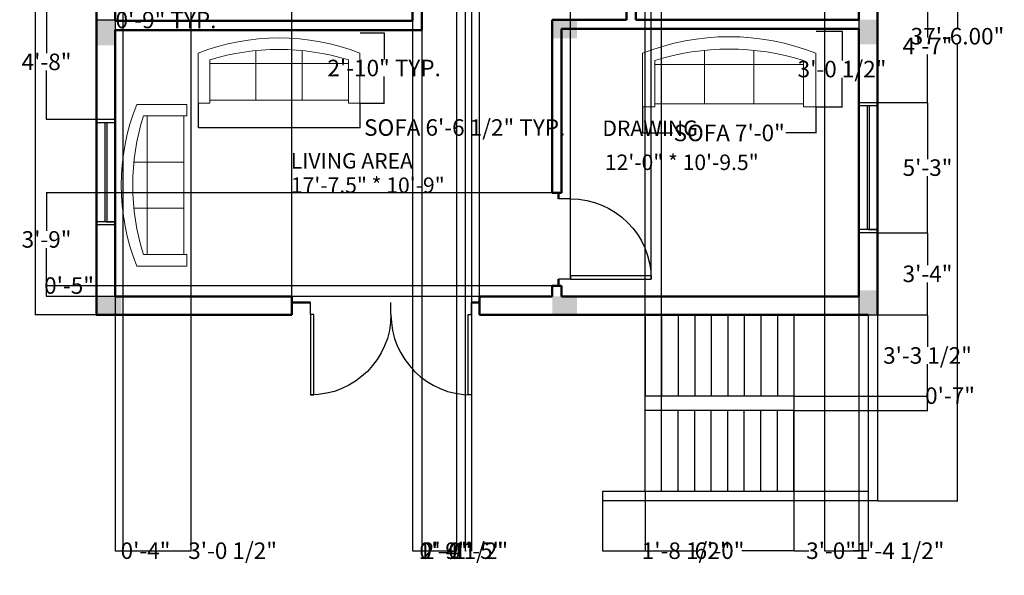
# Model space of a CAD drawing. Units: inches. Extents: x 9717 to 10218, y 17835 to 18358.
# Tile 1 of 4: x 9736 to 10212, y 17835 to 18104. Entities that reach past the tile are written whole.
import ezdxf

# ---------------------------------------------------------------- set-up
doc = ezdxf.new("R2010")
doc.units = ezdxf.units.IN
for name, color, linetype, lineweight in [('A-AREA-IDEN', 3, 'Continuous', 25), ('COLUMN', 7, 'Continuous', 35), ('DIMENSIONS', 3, 'Continuous', 18), ('DOORS', 1, 'Continuous', 25), ('FURNITURES', 2, 'Continuous', 18), ('STAIRS', 6, 'Continuous', 25), ('WALLS', 7, 'Continuous', 50), ('WINDOWS', 4, 'Continuous', 25)]:
    doc.layers.add(name, color=color, linetype=linetype, lineweight=lineweight)
doc.styles.get("Standard").update_dxf_attribs({"font": 'arial.ttf'})
doc.dimstyles.get("Standard").update_dxf_attribs({"dimtxt": 8, "dimasz": 0.18, "dimexe": 0.18, "dimexo": 0.0625, "dimgap": 0.09, "dimtad": 0, "dimtih": 1, "dimtoh": 1, "dimzin": 0, "dimdsep": 46, "dimlunit": 3, "dimtxsty": 'Standard', "dimcen": 0.09, "dimadec": 0, "dimazin": 0, "dimtfac": 1, "dimtofl": 0, "dimtmove": 0, "dimatfit": 3, "dimfxl": 1, "dimtolj": 1, "dimtzin": 0, "dimarcsym": 0})

# ---------------------------------------------------------------- blocks, each defined once
blk = doc.blocks.new('*U2')
for p, q in [((0, 0), (0, -6)), ((40, 0), (40, -6))]:
    blk.add_line(p, q)
blk.add_lwpolyline([(0, 0), (0, 40), (1.75, 40), (1.75, 0)], close=True)
blk.add_arc((0, 0), 40, 0, 90)
blk = doc.blocks.new('Sofa - Roundback 7 ft.')
for p, q in [((-12.00002, -32.4421), (-12.00003, -6.5971)), ((11.99997, -32.4421), (11.99998, -6.5971)), ((-36.000027, -34), (-36.000027, -11.4696)), ((-35.999844, -13.3819), (35.9998, -13.3819)), ((35.99998, -34), (35.99998, -11.4696)), ((-36.000027, -32.4421), (35.99998, -32.4421))]:
    blk.add_line(p, q)
for points in [[(-36.000027, -34), (-42.000027, -34), (-42.000027, -8)], [(41.99998, -8), (41.99998, -34), (35.99998, -34)]]:
    blk.add_lwpolyline(points)
for centre, radius, start, end in [((0, -114.25), 114.25, 68.43141, 111.5686), ((-0.00001, -127.1968), 121.1968, 72.72033, 107.2797)]:
    blk.add_arc(centre, radius, start, end)
blk = doc.blocks.new('*D9')
at = {"layer": 'Defpoints', "color": 0, "transparency": 16777216}
for p in [(9772.76, 18321.49), (9743.19, 17961.49), (9772.76, 17961.49)]:
    blk.add_point(p, dxfattribs=at)
at = {"layer": 'DIMENSIONS', "color": 0, "lineweight": -2, "transparency": 16777216}
for p, q in [((9772.7, 18321.49), (9743.01, 18321.49)), ((9743.19, 18321.31), (9743.19, 18145.67)), ((9743.19, 17961.67), (9743.19, 18137.31)), ((9772.7, 17961.49), (9743.01, 17961.49))]:
    blk.add_line(p, q, dxfattribs=at)
at = {"layer": 'DIMENSIONS', "color": 0, "transparency": 16777216}
for points in [[(9743.16, 18321.31), (9743.22, 18321.31), (9743.19, 18321.49)], [(9743.16, 17961.67), (9743.22, 17961.67), (9743.19, 17961.49)]]:
    blk.add_solid(points, dxfattribs=at)
at = {"layer": 'DIMENSIONS', "color": 0, "transparency": 16777216, "insert": (9743.19, 18141.49), "char_height": 8, "attachment_point": 5}
blk.add_mtext("\\A1;30'", dxfattribs=at)
blk = doc.blocks.new('*D10')
at = {"layer": 'Defpoints', "color": 0, "transparency": 16777216}
for p in [(10150.76, 18321.49), (10150.76, 17871.49), (10189.42, 17871.49)]:
    blk.add_point(p, dxfattribs=at)
at = {"layer": 'DIMENSIONS', "color": 0, "lineweight": -2, "transparency": 16777216}
for p, q in [((10150.82, 18321.49), (10189.6, 18321.49)), ((10189.42, 18321.31), (10189.42, 18100.67)), ((10189.42, 17871.67), (10189.42, 18092.31)), ((10150.82, 17871.49), (10189.6, 17871.49))]:
    blk.add_line(p, q, dxfattribs=at)
at = {"layer": 'DIMENSIONS', "color": 0, "transparency": 16777216}
for points in [[(10189.39, 18321.31), (10189.45, 18321.31), (10189.42, 18321.49)], [(10189.39, 17871.67), (10189.45, 17871.67), (10189.42, 17871.49)]]:
    blk.add_solid(points, dxfattribs=at)
at = {"layer": 'DIMENSIONS', "color": 0, "transparency": 16777216, "insert": (10189.42, 18096.49), "char_height": 8, "attachment_point": 5}
blk.add_mtext('\\A1;37\'-6.00"', dxfattribs=at)
blk = doc.blocks.new('WIN-48IN')
for p, q in [((0.5, 9), (0, 9)), ((0, 9), (0, 0)), ((1, 9), (0.5, 9)), ((1.5, 9), (1, 9)), ((1.5, 9), (1.5, 0)), ((1.5, 5), (49.5, 5)), ((49.5, 4.5), (49.5, 9)), ((49.5, 9), (49.5, 0)), ((49.5, 9), (51, 9)), ((51, 9), (51, 0)), ((0, 0), (1.5, 0)), ((1.5, 4), (49.5, 4)), ((51, 0), (49.5, 0))]:
    blk.add_line(p, q)
blk = doc.blocks.new('COL-12X9IN')
h = blk.add_hatch(color=256)
h.dxf.hatch_style = 1
h.paths.add_polyline_path([(12, 0), (12, 9), (0, 9), (0, 0)])
blk = doc.blocks.new('*D17')
at = {"layer": 'Defpoints', "color": 0, "transparency": 16777216}
for p in [(9772.76, 18112.01), (9781.76, 18112.01), (9781.76, 18104.36)]:
    blk.add_point(p, dxfattribs=at)
at = {"layer": 'DIMENSIONS', "color": 0, "lineweight": -2, "transparency": 16777216}
for p, q in [((9772.76, 18111.95), (9772.76, 18104.18)), ((9781.76, 18111.95), (9781.76, 18104.18)), ((9772.94, 18104.36), (9781.58, 18104.36)), ((9781.76, 18104.36), (9781.94, 18104.36))]:
    blk.add_line(p, q, dxfattribs=at)
at = {"layer": 'DIMENSIONS', "color": 0, "transparency": 16777216}
for points in [[(9772.94, 18104.39), (9772.94, 18104.33), (9772.76, 18104.36)], [(9781.58, 18104.39), (9781.58, 18104.33), (9781.76, 18104.36)]]:
    blk.add_solid(points, dxfattribs=at)
at = {"layer": 'DIMENSIONS', "color": 0, "transparency": 16777216, "insert": (9806.41, 18104.36), "char_height": 8, "attachment_point": 5}
blk.add_mtext('\\A1;0\'-9" TYP.', dxfattribs=at)
blk = doc.blocks.new('*D20')
at = {"layer": 'Defpoints', "color": 0, "transparency": 16777216}
for p in [(10036.94, 18062.24), (10120.94, 18062.24), (10120.94, 18049.64)]:
    blk.add_point(p, dxfattribs=at)
at = {"layer": 'DIMENSIONS', "color": 0, "lineweight": -2, "transparency": 16777216}
for p, q in [((10036.94, 18062.17), (10036.94, 18049.46)), ((10120.94, 18062.17), (10120.94, 18049.46)), ((10037.12, 18049.64), (10051.47, 18049.64)), ((10120.76, 18049.64), (10106.41, 18049.64))]:
    blk.add_line(p, q, dxfattribs=at)
at = {"layer": 'DIMENSIONS', "color": 0, "transparency": 16777216}
for points in [[(10037.12, 18049.67), (10037.12, 18049.61), (10036.94, 18049.64)], [(10120.76, 18049.67), (10120.76, 18049.61), (10120.94, 18049.64)]]:
    blk.add_solid(points, dxfattribs=at)
at = {"layer": 'DIMENSIONS', "color": 0, "transparency": 16777216, "insert": (10078.94, 18049.64), "char_height": 8, "attachment_point": 5}
blk.add_mtext('\\A1;SOFA 7\'-0"', dxfattribs=at)
blk = doc.blocks.new('*D21')
at = {"layer": 'Defpoints', "color": 0, "transparency": 16777216}
for p in [(10120.94, 18098.9), (10133.54, 18098.9), (10120.94, 18062.24)]:
    blk.add_point(p, dxfattribs=at)
at = {"layer": 'DIMENSIONS', "color": 0, "lineweight": -2, "transparency": 16777216}
for p, q in [((10121, 18098.9), (10133.72, 18098.9)), ((10133.54, 18098.72), (10133.54, 18084.8)), ((10133.54, 18062.42), (10133.54, 18076.34)), ((10121, 18062.24), (10133.72, 18062.24))]:
    blk.add_line(p, q, dxfattribs=at)
at = {"layer": 'DIMENSIONS', "color": 0, "transparency": 16777216}
for points in [[(10133.51, 18098.72), (10133.57, 18098.72), (10133.54, 18098.9)], [(10133.51, 18062.42), (10133.57, 18062.42), (10133.54, 18062.24)]]:
    blk.add_solid(points, dxfattribs=at)
at = {"layer": 'DIMENSIONS', "color": 0, "transparency": 16777216, "insert": (10133.54, 18080.57), "char_height": 8, "attachment_point": 5}
blk.add_mtext('\\A1;3\'-0 1/2"', dxfattribs=at)
blk = doc.blocks.new('*D22')
at = {"layer": 'Defpoints', "color": 0, "transparency": 16777216}
for p in [(9821.99, 18064.01), (9900.24, 18064.01), (9900.24, 18052.27)]:
    blk.add_point(p, dxfattribs=at)
at = {"layer": 'DIMENSIONS', "color": 0, "lineweight": -2, "transparency": 16777216}
for p, q in [((9821.99, 18063.95), (9821.99, 18052.09)), ((9900.24, 18063.95), (9900.24, 18052.09)), ((9822.17, 18052.27), (9900.06, 18052.27)), ((9900.24, 18052.27), (9900.42, 18052.27))]:
    blk.add_line(p, q, dxfattribs=at)
at = {"layer": 'DIMENSIONS', "color": 0, "transparency": 16777216}
for points in [[(9822.17, 18052.3), (9822.17, 18052.24), (9821.99, 18052.27)], [(9900.06, 18052.3), (9900.06, 18052.24), (9900.24, 18052.27)]]:
    blk.add_solid(points, dxfattribs=at)
at = {"layer": 'DIMENSIONS', "color": 0, "transparency": 16777216, "insert": (9950.96, 18052.27), "char_height": 8, "attachment_point": 5}
blk.add_mtext('\\A1;SOFA 6\'-6 1/2" TYP.', dxfattribs=at)
blk = doc.blocks.new('*D23')
at = {"layer": 'Defpoints', "color": 0, "transparency": 16777216}
for p in [(9900.24, 18098.17), (9911.98, 18098.17), (9900.24, 18064.01)]:
    blk.add_point(p, dxfattribs=at)
at = {"layer": 'DIMENSIONS', "color": 0, "lineweight": -2, "transparency": 16777216}
for p, q in [((9900.31, 18098.17), (9912.16, 18098.17)), ((9911.98, 18097.99), (9911.98, 18085.27)), ((9911.98, 18064.19), (9911.98, 18076.92)), ((9900.31, 18064.01), (9912.16, 18064.01))]:
    blk.add_line(p, q, dxfattribs=at)
at = {"layer": 'DIMENSIONS', "color": 0, "transparency": 16777216}
for points in [[(9911.95, 18097.99), (9912.01, 18097.99), (9911.98, 18098.17)], [(9911.95, 18064.19), (9912.01, 18064.19), (9911.98, 18064.01)]]:
    blk.add_solid(points, dxfattribs=at)
at = {"layer": 'DIMENSIONS', "color": 0, "transparency": 16777216, "insert": (9911.98, 18081.09), "char_height": 8, "attachment_point": 5}
blk.add_mtext('\\A1;2\'-10" TYP.', dxfattribs=at)
blk = doc.blocks.new('*D32')
at = {"layer": 'Defpoints', "color": 0, "transparency": 16777216}
for p in [(9867.28, 18345.64), (9867.28, 17970.49), (9772.76, 17961.49)]:
    blk.add_point(p, dxfattribs=at)
at = {"layer": 'DIMENSIONS', "color": 0, "lineweight": -2, "transparency": 16777216}
for p, q in [((9772.76, 17961.55), (9772.76, 18345.82)), ((9772.94, 18345.64), (9796.9, 18345.64)), ((9867.1, 18345.64), (9843.14, 18345.64)), ((9867.28, 17970.55), (9867.28, 18345.82))]:
    blk.add_line(p, q, dxfattribs=at)
at = {"layer": 'DIMENSIONS', "color": 0, "transparency": 16777216}
for points in [[(9772.94, 18345.67), (9772.94, 18345.61), (9772.76, 18345.64)], [(9867.1, 18345.67), (9867.1, 18345.61), (9867.28, 18345.64)]]:
    blk.add_solid(points, dxfattribs=at)
at = {"layer": 'DIMENSIONS', "color": 0, "transparency": 16777216, "insert": (9820.02, 18345.64), "char_height": 8, "attachment_point": 5}
blk.add_mtext('\\A1;7\'-10 1/2"', dxfattribs=at)
blk = doc.blocks.new('*D33')
at = {"layer": 'Defpoints', "color": 0, "transparency": 16777216}
for p in [(9958.06, 18345.64), (9867.28, 17970.49), (9958.06, 17970.49)]:
    blk.add_point(p, dxfattribs=at)
at = {"layer": 'DIMENSIONS', "color": 0, "lineweight": -2, "transparency": 16777216}
for p, q in [((9867.28, 17970.55), (9867.28, 18345.82)), ((9867.46, 18345.64), (9901.98, 18345.64)), ((9957.88, 18345.64), (9923.36, 18345.64)), ((9958.06, 17970.55), (9958.06, 18345.82))]:
    blk.add_line(p, q, dxfattribs=at)
at = {"layer": 'DIMENSIONS', "color": 0, "transparency": 16777216}
for points in [[(9867.46, 18345.67), (9867.46, 18345.61), (9867.28, 18345.64)], [(9957.88, 18345.67), (9957.88, 18345.61), (9958.06, 18345.64)]]:
    blk.add_solid(points, dxfattribs=at)
at = {"layer": 'DIMENSIONS', "color": 0, "transparency": 16777216, "insert": (9912.67, 18345.64), "char_height": 8, "attachment_point": 5}
blk.add_mtext('\\A1;7\'-7"', dxfattribs=at)
blk = doc.blocks.new('*D34')
at = {"layer": 'Defpoints', "color": 0, "transparency": 16777216}
for p in [(10038.26, 17875.99), (10110.26, 17875.99), (10110.26, 17847.34)]:
    blk.add_point(p, dxfattribs=at)
at = {"layer": 'DIMENSIONS', "color": 0, "lineweight": -2, "transparency": 16777216}
for p, q in [((10038.26, 17875.93), (10038.26, 17847.16)), ((10110.26, 17875.93), (10110.26, 17847.16)), ((10038.44, 17847.34), (10063.52, 17847.34)), ((10110.08, 17847.34), (10085.01, 17847.34))]:
    blk.add_line(p, q, dxfattribs=at)
at = {"layer": 'DIMENSIONS', "color": 0, "transparency": 16777216}
for points in [[(10038.44, 17847.37), (10038.44, 17847.31), (10038.26, 17847.34)], [(10110.08, 17847.37), (10110.08, 17847.31), (10110.26, 17847.34)]]:
    blk.add_solid(points, dxfattribs=at)
at = {"layer": 'DIMENSIONS', "color": 0, "transparency": 16777216, "insert": (10074.26, 17847.34), "char_height": 8, "attachment_point": 5}
blk.add_mtext('\\A1;6\'-0"', dxfattribs=at)
blk = doc.blocks.new('*D35')
at = {"layer": 'Defpoints', "color": 0, "transparency": 16777216}
for p in [(10110.26, 17875.99), (10146.26, 17875.99), (10146.26, 17847.34)]:
    blk.add_point(p, dxfattribs=at)
at = {"layer": 'DIMENSIONS', "color": 0, "lineweight": -2, "transparency": 16777216}
for p, q in [((10110.26, 17875.93), (10110.26, 17847.16)), ((10146.26, 17875.93), (10146.26, 17847.16)), ((10110.44, 17847.34), (10117.54, 17847.34)), ((10146.08, 17847.34), (10138.98, 17847.34))]:
    blk.add_line(p, q, dxfattribs=at)
at = {"layer": 'DIMENSIONS', "color": 0, "transparency": 16777216}
for points in [[(10110.44, 17847.37), (10110.44, 17847.31), (10110.26, 17847.34)], [(10146.08, 17847.37), (10146.08, 17847.31), (10146.26, 17847.34)]]:
    blk.add_solid(points, dxfattribs=at)
at = {"layer": 'DIMENSIONS', "color": 0, "transparency": 16777216, "insert": (10128.26, 17847.34), "char_height": 8, "attachment_point": 5}
blk.add_mtext('\\A1;3\'-0"', dxfattribs=at)
blk = doc.blocks.new('*D36')
at = {"layer": 'Defpoints', "color": 0, "transparency": 16777216}
for p in [(10038.26, 17875.99), (10017.58, 17871.49), (10038.26, 17847.34)]:
    blk.add_point(p, dxfattribs=at)
at = {"layer": 'DIMENSIONS', "color": 0, "lineweight": -2, "transparency": 16777216}
for p, q in [((10038.26, 17875.93), (10038.26, 17847.16)), ((10017.58, 17871.43), (10017.58, 17847.16)), ((10017.76, 17847.34), (10038.08, 17847.34)), ((10038.26, 17847.34), (10038.44, 17847.34))]:
    blk.add_line(p, q, dxfattribs=at)
at = {"layer": 'DIMENSIONS', "color": 0, "transparency": 16777216}
for points in [[(10017.76, 17847.37), (10017.76, 17847.31), (10017.58, 17847.34)], [(10038.08, 17847.37), (10038.08, 17847.31), (10038.26, 17847.34)]]:
    blk.add_solid(points, dxfattribs=at)
at = {"layer": 'DIMENSIONS', "color": 0, "transparency": 16777216, "insert": (10058.11, 17847.34), "char_height": 8, "attachment_point": 5}
blk.add_mtext('\\A1;1\'-8 1/2"', dxfattribs=at)
blk = doc.blocks.new('*D37')
at = {"layer": 'Defpoints', "color": 0, "transparency": 16777216}
for p in [(10110.26, 17961.49), (10110.26, 17922.24), (10174.91, 17922.24)]:
    blk.add_point(p, dxfattribs=at)
at = {"layer": 'DIMENSIONS', "color": 0, "lineweight": -2, "transparency": 16777216}
for p, q in [((10110.32, 17961.49), (10175.09, 17961.49)), ((10174.91, 17961.31), (10174.91, 17946.1)), ((10174.91, 17922.42), (10174.91, 17937.64)), ((10110.32, 17922.24), (10175.09, 17922.24))]:
    blk.add_line(p, q, dxfattribs=at)
at = {"layer": 'DIMENSIONS', "color": 0, "transparency": 16777216}
for points in [[(10174.88, 17961.31), (10174.94, 17961.31), (10174.91, 17961.49)], [(10174.88, 17922.42), (10174.94, 17922.42), (10174.91, 17922.24)]]:
    blk.add_solid(points, dxfattribs=at)
at = {"layer": 'DIMENSIONS', "color": 0, "transparency": 16777216, "insert": (10174.91, 17941.87), "char_height": 8, "attachment_point": 5}
blk.add_mtext('\\A1;3\'-3 1/2"', dxfattribs=at)
blk = doc.blocks.new('*D38')
at = {"layer": 'Defpoints', "color": 0, "transparency": 16777216}
for p in [(10110.260349, 17922.241492), (10174.910349, 17922.241492), (10110.260349, 17915.241492)]:
    blk.add_point(p, dxfattribs=at)
at = {"layer": 'DIMENSIONS', "color": 0, "lineweight": -2, "transparency": 16777216}
for p, q in [((10110.322849, 17922.241492), (10175.090349, 17922.241492)), ((10174.910349, 17922.241492), (10174.910349, 17922.421492)), ((10174.910349, 17922.421492), (10175.090349, 17922.421492)), ((10174.910349, 17915.421492), (10174.910349, 17922.061492)), ((10110.322849, 17915.241492), (10175.090349, 17915.241492))]:
    blk.add_line(p, q, dxfattribs=at)
at = {"layer": 'DIMENSIONS', "color": 0, "transparency": 16777216}
for points in [[(10174.880349, 17922.061492), (10174.940349, 17922.061492), (10174.910349, 17922.241492)], [(10174.880349, 17915.421492), (10174.940349, 17915.421492), (10174.910349, 17915.241492)]]:
    blk.add_solid(points, dxfattribs=at)
at = {"layer": 'DIMENSIONS', "color": 0, "transparency": 16777216, "insert": (10185.813364, 17922.421492), "char_height": 8, "attachment_point": 5}
blk.add_mtext('\\A1;0\'-7"', dxfattribs=at)
blk = doc.blocks.new('*D39')
at = {"layer": 'Defpoints', "color": 0, "transparency": 16777216}
for p in [(10046.260349, 18345.641492), (10038.260349, 17915.241492), (10046.260349, 17915.241492)]:
    blk.add_point(p, dxfattribs=at)
at = {"layer": 'DIMENSIONS', "color": 0, "lineweight": -2, "transparency": 16777216}
for p, q in [((10038.260349, 17915.303992), (10038.260349, 18345.821492)), ((10038.440349, 18345.641492), (10046.080349, 18345.641492)), ((10046.260349, 17915.303992), (10046.260349, 18345.821492)), ((10046.260349, 18345.641492), (10046.440349, 18345.641492))]:
    blk.add_line(p, q, dxfattribs=at)
at = {"layer": 'DIMENSIONS', "color": 0, "transparency": 16777216}
for points in [[(10038.440349, 18345.671492), (10038.440349, 18345.611492), (10038.260349, 18345.641492)], [(10046.080349, 18345.671492), (10046.080349, 18345.611492), (10046.260349, 18345.641492)]]:
    blk.add_solid(points, dxfattribs=at)
at = {"layer": 'DIMENSIONS', "color": 0, "transparency": 16777216, "insert": (10057.163364, 18345.641492), "char_height": 8, "attachment_point": 5}
blk.add_mtext('\\A1;0\'-8"', dxfattribs=at)
blk = doc.blocks.new('*D40')
at = {"layer": 'Defpoints', "color": 0, "transparency": 16777216}
for p in [(9781.76, 18312.49), (9818.43, 18312.49), (9818.43, 17847.34)]:
    blk.add_point(p, dxfattribs=at)
at = {"layer": 'DIMENSIONS', "color": 0, "lineweight": -2, "transparency": 16777216}
for p, q in [((9781.76, 18312.43), (9781.76, 17847.16)), ((9818.43, 18312.43), (9818.43, 17847.16)), ((9781.94, 17847.34), (9818.25, 17847.34)), ((9818.43, 17847.34), (9818.61, 17847.34))]:
    blk.add_line(p, q, dxfattribs=at)
at = {"layer": 'DIMENSIONS', "color": 0, "transparency": 16777216}
for points in [[(9781.94, 17847.37), (9781.94, 17847.31), (9781.76, 17847.34)], [(9818.25, 17847.37), (9818.25, 17847.31), (9818.43, 17847.34)]]:
    blk.add_solid(points, dxfattribs=at)
at = {"layer": 'DIMENSIONS', "color": 0, "transparency": 16777216, "insert": (9838.65, 17847.34), "char_height": 8, "attachment_point": 5}
blk.add_mtext('\\A1;3\'-0 1/2"', dxfattribs=at)
blk = doc.blocks.new('*D41')
at = {"layer": 'Defpoints', "color": 0, "transparency": 16777216}
for p in [(9930.26, 18312.49), (9947.05, 18312.49), (9947.05, 17847.34)]:
    blk.add_point(p, dxfattribs=at)
at = {"layer": 'DIMENSIONS', "color": 0, "lineweight": -2, "transparency": 16777216}
for p, q in [((9930.26, 18312.43), (9930.26, 17847.16)), ((9947.05, 18312.43), (9947.05, 17847.16)), ((9930.44, 17847.34), (9946.87, 17847.34)), ((9947.05, 17847.34), (9947.23, 17847.34))]:
    blk.add_line(p, q, dxfattribs=at)
at = {"layer": 'DIMENSIONS', "color": 0, "transparency": 16777216}
for points in [[(9930.44, 17847.37), (9930.44, 17847.31), (9930.26, 17847.34)], [(9946.87, 17847.37), (9946.87, 17847.31), (9947.05, 17847.34)]]:
    blk.add_solid(points, dxfattribs=at)
at = {"layer": 'DIMENSIONS', "color": 0, "transparency": 16777216, "insert": (9957.58, 17847.34), "char_height": 8, "attachment_point": 5}
blk.add_mtext('\\A1;1\'-5"', dxfattribs=at)
blk = doc.blocks.new('*D44')
at = {"layer": 'Defpoints', "color": 0, "transparency": 16777216}
for p in [(9748.61, 18112.01), (9772.76, 18112.01), (9772.76, 18056.11)]:
    blk.add_point(p, dxfattribs=at)
at = {"layer": 'DIMENSIONS', "color": 0, "lineweight": -2, "transparency": 16777216}
for p, q in [((9772.7, 18112.01), (9748.43, 18112.01)), ((9748.61, 18111.83), (9748.61, 18088.23)), ((9748.61, 18056.29), (9748.61, 18079.88)), ((9772.7, 18056.11), (9748.43, 18056.11))]:
    blk.add_line(p, q, dxfattribs=at)
at = {"layer": 'DIMENSIONS', "color": 0, "transparency": 16777216}
for points in [[(9748.58, 18111.83), (9748.64, 18111.83), (9748.61, 18112.01)], [(9748.58, 18056.29), (9748.64, 18056.29), (9748.61, 18056.11)]]:
    blk.add_solid(points, dxfattribs=at)
at = {"layer": 'DIMENSIONS', "color": 0, "transparency": 16777216, "insert": (9748.61, 18084.06), "char_height": 8, "attachment_point": 5}
blk.add_mtext('\\A1;4\'-8"', dxfattribs=at)
blk = doc.blocks.new('*D45')
at = {"layer": 'Defpoints', "color": 0, "transparency": 16777216}
for p in [(10150.76, 18001.34), (10174.91, 18001.34), (10150.76, 17961.49)]:
    blk.add_point(p, dxfattribs=at)
at = {"layer": 'DIMENSIONS', "color": 0, "lineweight": -2, "transparency": 16777216}
for p, q in [((10150.82, 18001.34), (10175.09, 18001.34)), ((10174.91, 18001.16), (10174.91, 17985.59)), ((10174.91, 17961.67), (10174.91, 17977.24)), ((10150.82, 17961.49), (10175.09, 17961.49))]:
    blk.add_line(p, q, dxfattribs=at)
at = {"layer": 'DIMENSIONS', "color": 0, "transparency": 16777216}
for points in [[(10174.88, 18001.16), (10174.94, 18001.16), (10174.91, 18001.34)], [(10174.88, 17961.67), (10174.94, 17961.67), (10174.91, 17961.49)]]:
    blk.add_solid(points, dxfattribs=at)
at = {"layer": 'DIMENSIONS', "color": 0, "transparency": 16777216, "insert": (10174.91, 17981.42), "char_height": 8, "attachment_point": 5}
blk.add_mtext('\\A1;3\'-4"', dxfattribs=at)
blk = doc.blocks.new('*D46')
at = {"layer": 'Defpoints', "color": 0, "transparency": 16777216}
for p in [(10150.76, 18064.34), (10174.91, 18064.34), (10150.76, 18001.34)]:
    blk.add_point(p, dxfattribs=at)
at = {"layer": 'DIMENSIONS', "color": 0, "lineweight": -2, "transparency": 16777216}
for p, q in [((10150.82, 18064.34), (10175.09, 18064.34)), ((10174.91, 18064.16), (10174.91, 18037.02)), ((10174.91, 18001.52), (10174.91, 18028.66)), ((10150.82, 18001.34), (10175.09, 18001.34))]:
    blk.add_line(p, q, dxfattribs=at)
at = {"layer": 'DIMENSIONS', "color": 0, "transparency": 16777216}
for points in [[(10174.88, 18064.16), (10174.94, 18064.16), (10174.91, 18064.34)], [(10174.88, 18001.52), (10174.94, 18001.52), (10174.91, 18001.34)]]:
    blk.add_solid(points, dxfattribs=at)
at = {"layer": 'DIMENSIONS', "color": 0, "transparency": 16777216, "insert": (10174.91, 18032.84), "char_height": 8, "attachment_point": 5}
blk.add_mtext('\\A1;5\'-3"', dxfattribs=at)
blk = doc.blocks.new('*D47')
at = {"layer": 'Defpoints', "color": 0, "transparency": 16777216}
for p in [(10150.76, 18119.16), (10174.91, 18119.16), (10150.76, 18064.34)]:
    blk.add_point(p, dxfattribs=at)
at = {"layer": 'DIMENSIONS', "color": 0, "lineweight": -2, "transparency": 16777216}
for p, q in [((10150.82, 18119.16), (10175.09, 18119.16)), ((10174.91, 18118.98), (10174.91, 18095.84)), ((10174.91, 18064.52), (10174.91, 18087.66)), ((10150.82, 18064.34), (10175.09, 18064.34))]:
    blk.add_line(p, q, dxfattribs=at)
at = {"layer": 'DIMENSIONS', "color": 0, "transparency": 16777216}
for points in [[(10174.88, 18118.98), (10174.94, 18118.98), (10174.91, 18119.16)], [(10174.88, 18064.52), (10174.94, 18064.52), (10174.91, 18064.34)]]:
    blk.add_solid(points, dxfattribs=at)
at = {"layer": 'DIMENSIONS', "color": 0, "transparency": 16777216, "insert": (10174.91, 18091.75), "char_height": 8, "attachment_point": 5}
blk.add_mtext('\\A1;4\'-7"', dxfattribs=at)
blk = doc.blocks.new('*D54')
at = {"layer": 'Defpoints', "color": 0, "transparency": 16777216}
for p in [(9748.61, 18020.62), (9993.26, 18020.62), (9993.26, 17975.56)]:
    blk.add_point(p, dxfattribs=at)
at = {"layer": 'DIMENSIONS', "color": 0, "lineweight": -2, "transparency": 16777216}
for p, q in [((9993.2, 18020.62), (9748.43, 18020.62)), ((9748.61, 18020.44), (9748.61, 18002.27)), ((9748.61, 17975.74), (9748.61, 17993.91)), ((9993.2, 17975.56), (9748.43, 17975.56))]:
    blk.add_line(p, q, dxfattribs=at)
at = {"layer": 'DIMENSIONS', "color": 0, "transparency": 16777216}
for points in [[(9748.58, 18020.44), (9748.64, 18020.44), (9748.61, 18020.62)], [(9748.58, 17975.74), (9748.64, 17975.74), (9748.61, 17975.56)]]:
    blk.add_solid(points, dxfattribs=at)
at = {"layer": 'DIMENSIONS', "color": 0, "transparency": 16777216, "insert": (9748.61, 17998.09), "char_height": 8, "attachment_point": 5}
blk.add_mtext('\\A1;3\'-9"', dxfattribs=at)
blk = doc.blocks.new('*D55')
at = {"layer": 'Defpoints', "color": 0, "transparency": 16777216}
for p in [(9925.76, 18103.99), (9930.26, 18099.49), (9930.26, 17847.34)]:
    blk.add_point(p, dxfattribs=at)
at = {"layer": 'DIMENSIONS', "color": 0, "lineweight": -2, "transparency": 16777216}
for p, q in [((9925.76, 18103.93), (9925.76, 17847.16)), ((9930.26, 18099.43), (9930.26, 17847.16)), ((9925.94, 17847.34), (9930.08, 17847.34)), ((9930.26, 17847.34), (9930.44, 17847.34))]:
    blk.add_line(p, q, dxfattribs=at)
at = {"layer": 'DIMENSIONS', "color": 0, "transparency": 16777216}
for points in [[(9925.94, 17847.37), (9925.94, 17847.31), (9925.76, 17847.34)], [(9930.08, 17847.37), (9930.08, 17847.31), (9930.26, 17847.34)]]:
    blk.add_solid(points, dxfattribs=at)
at = {"layer": 'DIMENSIONS', "color": 0, "transparency": 16777216, "insert": (9950.48, 17847.34), "char_height": 8, "attachment_point": 5}
blk.add_mtext('\\A1;0\'-4 1/2"', dxfattribs=at)
blk = doc.blocks.new('*D57')
at = {"layer": 'Defpoints', "color": 0, "transparency": 16777216}
for p in [(10041.19, 18345.64), (10002.19, 17978.77), (10041.19, 17978.77)]:
    blk.add_point(p, dxfattribs=at)
at = {"layer": 'DIMENSIONS', "color": 0, "lineweight": -2, "transparency": 16777216}
for p, q in [((10002.19, 17978.83), (10002.19, 18345.82)), ((10002.37, 18345.64), (10010.97, 18345.64)), ((10041.01, 18345.64), (10032.41, 18345.64)), ((10041.19, 17978.83), (10041.19, 18345.82))]:
    blk.add_line(p, q, dxfattribs=at)
at = {"layer": 'DIMENSIONS', "color": 0, "transparency": 16777216}
for points in [[(10002.37, 18345.67), (10002.37, 18345.61), (10002.19, 18345.64)], [(10041.01, 18345.67), (10041.01, 18345.61), (10041.19, 18345.64)]]:
    blk.add_solid(points, dxfattribs=at)
at = {"layer": 'DIMENSIONS', "color": 0, "transparency": 16777216, "insert": (10021.69, 18345.64), "char_height": 8, "attachment_point": 5}
blk.add_mtext('\\A1;3\'-3"', dxfattribs=at)
blk = doc.blocks.new('*D58')
at = {"layer": 'Defpoints', "color": 0, "transparency": 16777216}
for p in [(9930.26, 18232.99), (9954.27, 18232.99), (9954.27, 17847.34)]:
    blk.add_point(p, dxfattribs=at)
at = {"layer": 'DIMENSIONS', "color": 0, "lineweight": -2, "transparency": 16777216}
for p, q in [((9930.26, 18232.93), (9930.26, 17847.16)), ((9954.27, 18232.93), (9954.27, 17847.16)), ((9930.44, 17847.34), (9931.48, 17847.34)), ((9954.09, 17847.34), (9953.06, 17847.34))]:
    blk.add_line(p, q, dxfattribs=at)
at = {"layer": 'DIMENSIONS', "color": 0, "transparency": 16777216}
for points in [[(9930.44, 17847.37), (9930.44, 17847.31), (9930.26, 17847.34)], [(9954.09, 17847.37), (9954.09, 17847.31), (9954.27, 17847.34)]]:
    blk.add_solid(points, dxfattribs=at)
at = {"layer": 'DIMENSIONS', "color": 0, "transparency": 16777216, "insert": (9942.27, 17847.34), "char_height": 8, "attachment_point": 5}
blk.add_mtext('\\A1;2\'-0"', dxfattribs=at)
blk = doc.blocks.new('*D60')
at = {"layer": 'Defpoints', "color": 0, "transparency": 16777216}
for p in [(9748.610349, 17975.563094), (9993.260349, 17975.563094), (9993.260349, 17970.491492)]:
    blk.add_point(p, dxfattribs=at)
at = {"layer": 'DIMENSIONS', "color": 0, "lineweight": -2, "transparency": 16777216}
for p, q in [((9993.197849, 17975.563094), (9748.430349, 17975.563094)), ((9748.610349, 17975.563094), (9748.610349, 17975.743094)), ((9748.610349, 17975.743094), (9748.790349, 17975.743094)), ((9748.610349, 17970.671492), (9748.610349, 17975.383094)), ((9993.197849, 17970.491492), (9748.430349, 17970.491492))]:
    blk.add_line(p, q, dxfattribs=at)
at = {"layer": 'DIMENSIONS', "color": 0, "transparency": 16777216}
for points in [[(9748.580349, 17975.383094), (9748.640349, 17975.383094), (9748.610349, 17975.563094)], [(9748.580349, 17970.671492), (9748.640349, 17970.671492), (9748.610349, 17970.491492)]]:
    blk.add_solid(points, dxfattribs=at)
at = {"layer": 'DIMENSIONS', "color": 0, "transparency": 16777216, "insert": (9759.513364, 17975.743094), "char_height": 8, "attachment_point": 5}
blk.add_mtext('\\A1;0\'-5"', dxfattribs=at)
blk = doc.blocks.new('*D62')
at = {"layer": 'Defpoints', "color": 0, "transparency": 16777216}
for p in [(9785.597893, 18202.734969), (9781.760349, 18192.491492), (9785.597893, 17847.341492)]:
    blk.add_point(p, dxfattribs=at)
at = {"layer": 'DIMENSIONS', "color": 0, "lineweight": -2, "transparency": 16777216}
for p, q in [((9785.597893, 18202.672469), (9785.597893, 17847.161492)), ((9781.760349, 18192.428992), (9781.760349, 17847.161492)), ((9781.940349, 17847.341492), (9785.417893, 17847.341492)), ((9785.597893, 17847.341492), (9785.777893, 17847.341492))]:
    blk.add_line(p, q, dxfattribs=at)
at = {"layer": 'DIMENSIONS', "color": 0, "transparency": 16777216}
for points in [[(9781.940349, 17847.371492), (9781.940349, 17847.311492), (9781.760349, 17847.341492)], [(9785.417893, 17847.371492), (9785.417893, 17847.311492), (9785.597893, 17847.341492)]]:
    blk.add_solid(points, dxfattribs=at)
at = {"layer": 'DIMENSIONS', "color": 0, "transparency": 16777216, "insert": (9796.500908, 17847.341492), "char_height": 8, "attachment_point": 5}
blk.add_mtext('\\A1;0\'-4"', dxfattribs=at)
blk = doc.blocks.new('*D64')
at = {"layer": 'Defpoints', "color": 0, "transparency": 16777216}
for p in [(9930.26, 18312.49), (9951.25, 18309.85), (9951.25, 17847.34)]:
    blk.add_point(p, dxfattribs=at)
at = {"layer": 'DIMENSIONS', "color": 0, "lineweight": -2, "transparency": 16777216}
for p, q in [((9930.26, 18312.43), (9930.26, 17847.16)), ((9951.25, 18309.78), (9951.25, 17847.16)), ((9930.08, 17847.34), (9929.9, 17847.34)), ((9951.43, 17847.34), (9951.61, 17847.34))]:
    blk.add_line(p, q, dxfattribs=at)
at = {"layer": 'DIMENSIONS', "color": 0, "transparency": 16777216}
for points in [[(9930.08, 17847.37), (9930.08, 17847.31), (9930.26, 17847.34)], [(9951.43, 17847.37), (9951.43, 17847.31), (9951.25, 17847.34)]]:
    blk.add_solid(points, dxfattribs=at)
at = {"layer": 'DIMENSIONS', "color": 0, "transparency": 16777216, "insert": (9940.75, 17847.34), "char_height": 8, "attachment_point": 5}
blk.add_mtext('\\A1;1\'-9"', dxfattribs=at)
blk = doc.blocks.new('*D65')
at = {"layer": 'Defpoints', "color": 0, "transparency": 16777216}
for p in [(10125.09, 18151.74), (10141.76, 18146.16), (10141.76, 17847.34)]:
    blk.add_point(p, dxfattribs=at)
at = {"layer": 'DIMENSIONS', "color": 0, "lineweight": -2, "transparency": 16777216}
for p, q in [((10125.09, 18151.67), (10125.09, 17847.16)), ((10141.76, 18146.09), (10141.76, 17847.16)), ((10125.27, 17847.34), (10141.58, 17847.34)), ((10141.76, 17847.34), (10141.94, 17847.34))]:
    blk.add_line(p, q, dxfattribs=at)
at = {"layer": 'DIMENSIONS', "color": 0, "transparency": 16777216}
for points in [[(10125.27, 17847.37), (10125.27, 17847.31), (10125.09, 17847.34)], [(10141.58, 17847.37), (10141.58, 17847.31), (10141.76, 17847.34)]]:
    blk.add_solid(points, dxfattribs=at)
at = {"layer": 'DIMENSIONS', "color": 0, "transparency": 16777216, "insert": (10161.61, 17847.34), "char_height": 8, "attachment_point": 5}
blk.add_mtext('\\A1;1\'-4 1/2"', dxfattribs=at)

msp = doc.modelspace()

# ---------------------------------------------------------------- linework, layer by layer
at = {"layer": 'STAIRS'}
for p, q in [((10038.26, 17961.491), (10038.26, 17922.241)), ((10046.26, 17961.491), (10046.26, 17922.241)), ((10054.26, 17961.491), (10054.26, 17922.241)), ((10062.26, 17961.491), (10062.26, 17922.241)), ((10070.26, 17961.491), (10070.26, 17922.241)), ((10078.26, 17961.491), (10078.26, 17922.241)), ((10086.26, 17961.491), (10086.26, 17922.241)), ((10094.26, 17961.491), (10094.26, 17922.241)), ((10102.26, 17961.491), (10102.26, 17922.241)), ((10110.26, 17961.491), (10110.26, 17915.241)), ((10146.26, 17961.491), (10146.26, 17875.991)), ((10150.76, 17961.491), (10150.76, 17871.491)), ((10110.26, 17922.241), (10038.26, 17922.241)), ((10110.26, 17915.241), (10038.26, 17915.241)), ((10038.26, 17875.991), (10038.26, 17915.241)), ((10046.26, 17875.991), (10046.26, 17915.241)), ((10054.26, 17875.991), (10054.26, 17915.241)), ((10062.26, 17875.991), (10062.26, 17915.241)), ((10070.26, 17875.991), (10070.26, 17915.241)), ((10078.26, 17875.991), (10078.26, 17915.241)), ((10086.26, 17875.991), (10086.26, 17915.241)), ((10094.26, 17875.991), (10094.26, 17915.241)), ((10102.26, 17875.991), (10102.26, 17915.241)), ((10110.26, 17915.241), (10110.26, 17875.991)), ((10110.26, 17875.991), (10110.26, 17915.241)), ((10146.26, 17875.991), (10017.581, 17875.991)), ((10017.581, 17875.991), (10017.581, 17871.491)), ((10150.76, 17871.491), (10017.581, 17871.491))]:
    msp.add_line(p, q, dxfattribs=at)
at = {"layer": 'WALLS'}
for p, q in [((9925.76, 18103.991), (9925.76, 18192.491)), ((9930.26, 18099.491), (9930.26, 18192.491)), ((9781.76, 18103.991), (9781.76, 18187.991)), ((10029.26, 18164.491), (10029.26, 18104.491)), ((10033.76, 18164.491), (10033.76, 18104.491)), ((10141.76, 18164.491), (10141.76, 18104.491)), ((9781.76, 18103.991), (9925.76, 18103.991)), ((9993.26, 18104.491), (10029.26, 18104.491)), ((9993.26, 18104.491), (9993.26, 18020.621)), ((10033.76, 18104.491), (10141.76, 18104.491)), ((9781.76, 17970.491), (9781.76, 18099.491)), ((9781.76, 18099.491), (9930.26, 18099.491)), ((9997.76, 18099.991), (10141.76, 18099.991)), ((9997.76, 18099.991), (9997.76, 18020.621)), ((10141.76, 18099.991), (10141.76, 17970.491)), ((9997.76, 18020.621), (9993.26, 18020.621)), ((9996.337, 18017.769), (9996.337, 18020.621)), ((9996.337, 17978.769), (9996.337, 17975.563)), ((9993.26, 17975.563), (9997.76, 17975.563)), ((9993.26, 17975.563), (9993.26, 17970.491)), ((9997.76, 17975.563), (9997.76, 17970.491)), ((9867.276, 17970.491), (9781.76, 17970.491)), ((9867.276, 17970.491), (9867.276, 17961.491)), ((9876.293, 17967.603), (9867.276, 17967.603)), ((9954.293, 17967.603), (9958.06, 17967.603)), ((9993.26, 17970.491), (9958.06, 17970.491)), ((9958.06, 17961.491), (9958.06, 17970.491)), ((10141.76, 17970.491), (9997.76, 17970.491))]:
    msp.add_line(p, q, dxfattribs=at)
for points in [[(9867.276, 17961.491), (9772.76, 17961.491), (9772.76, 18321.491), (10150.76, 18321.491), (10150.76, 17961.491)], [(9915.294, 17961.491), (9915.292, 17961.491)], [(10146.26, 17961.491), (9958.06, 17961.491)]]:
    msp.add_lwpolyline(points, dxfattribs=at)
at = {"layer": 'WINDOWS'}
for p, q in [((10141.76, 18064.339), (10150.76, 18064.339)), ((10141.76, 18062.839), (10141.76, 18064.339)), ((10150.76, 18062.839), (10141.76, 18062.839)), ((10145.76, 18062.839), (10145.76, 18002.839)), ((10146.76, 18062.839), (10146.76, 18002.839)), ((10150.76, 18064.339), (10150.76, 18062.839)), ((10150.76, 18002.839), (10141.76, 18002.839)), ((10141.76, 18001.339), (10141.76, 18002.839)), ((10150.76, 18001.339), (10141.76, 18001.339)), ((10146.26, 18002.839), (10150.76, 18002.839)), ((10150.76, 18002.839), (10150.76, 18001.339))]:
    msp.add_line(p, q, dxfattribs=at)

# ---------------------------------------------------------------- block references
at = {"layer": 'COLUMN'}
for p, rotation in [((9772.76, 18104.016), 269.9999999999769), ((10141.76, 18104.492), 269.9999999999907), ((10141.76, 17973.482), 269.9999999999769)]:
    msp.add_blockref('COL-12X9IN', p, dxfattribs=dict(at, rotation=rotation))
for p in [(9993.316, 18095.483), (9772.816, 17961.559), (9993.316, 17961.483)]:
    msp.add_blockref('COL-12X9IN', p, dxfattribs=at)
at = {"layer": 'DOORS', "yscale": 0.975, "zscale": 0.975}
for p, xscale, rotation in [((10002.187, 17978.769), -0.975, 270), ((9876.293, 17961.753), -0.975, 180), ((9954.293, 17961.753), 0.975, 180)]:
    msp.add_blockref('*U2', p, dxfattribs=dict(at, xscale=xscale, rotation=rotation))
at = {"layer": 'FURNITURES', "xscale": 0.931560362652387, "yscale": 0.931560362652387, "zscale": 0.931560362652387}
msp.add_blockref('Sofa - Roundback 7 ft.', (9861.118, 18095.685), dxfattribs=at)
at = {"layer": 'FURNITURES'}
msp.add_blockref('Sofa - Roundback 7 ft.', (10078.937, 18096.236), dxfattribs=at)
at = {"layer": 'FURNITURES', "xscale": 0.931560362652387, "yscale": 0.931560362652387, "zscale": 0.931560362652387, "rotation": 90}
msp.add_blockref('Sofa - Roundback 7 ft.', (9784.772, 18024.322), dxfattribs=at)
at = {"layer": 'WINDOWS', "rotation": 270.0000000000058}
msp.add_blockref('WIN-48IN', (9772.76, 18056.109), dxfattribs=at)

# ---------------------------------------------------------------- texts
at = {"layer": 'A-AREA-IDEN'}
for s, p in [('DRAWING', (10017.586, 18048.166)), ('LIVING AREA', (9866.78, 18032.395)), ('12\'-0" * 10\'-9.5"', (10018.783, 18031.681)), ('17\'-7.5" * 10\'-9"', (9866.843, 18020.593))]:
    msp.add_text(s, height=7.5, dxfattribs=at).set_placement(p)

# ---------------------------------------------------------------- dimensions: what is measured, and where the dimension line sits
at = {"layer": 'DIMENSIONS'}
for base, p1, p2, picture, middle in [((9867.276, 18345.641), (9772.76, 17961.491), (9867.276, 17970.491), '*D32', (9820.018, 18345.641)), ((9958.06, 18345.641), (9867.276, 17970.491), (9958.06, 17970.491), '*D33', (9912.668, 18345.641)), ((10041.187, 18345.641), (10002.187, 17978.769), (10041.187, 17978.769), '*D57', (10021.687, 18345.641)), ((10046.26, 18345.641), (10038.26, 17915.241), (10046.26, 17915.241), '*D39', (10057.163, 18345.641)), ((9818.425, 17847.341), (9781.76, 18312.491), (9818.425, 18312.491), '*D40', (9838.646, 17847.341)), ((9951.246, 17847.341), (9930.26, 18312.491), (9951.246, 18309.847), '*D64', (9940.753, 17847.341)), ((9947.053, 17847.341), (9930.26, 18312.491), (9947.053, 18312.491), '*D41', (9957.579, 17847.341)), ((9954.275, 17847.341), (9930.26, 18232.991), (9954.275, 18232.991), '*D58', (9942.268, 17847.341)), ((9785.598, 17847.341), (9781.76, 18192.491), (9785.598, 18202.735), '*D62', (9796.501, 17847.341)), ((10141.76, 17847.341), (10125.095, 18151.737), (10141.76, 18146.155), '*D65', (10161.607, 17847.341)), ((9930.26, 17847.341), (9925.76, 18103.991), (9930.26, 18099.491), '*D55', (9950.484, 17847.341)), ((10038.26, 17847.341), (10017.581, 17871.491), (10038.26, 17875.991), '*D36', (10058.107, 17847.341)), ((10110.26, 17847.341), (10038.26, 17875.991), (10110.26, 17875.991), '*D34', (10074.26, 17847.341)), ((10146.26, 17847.341), (10110.26, 17875.991), (10146.26, 17875.991), '*D35', (10128.26, 17847.341))]:
    dim = msp.add_linear_dim(base=base, p1=p1, p2=p2, dimstyle='Standard', override={"dimdec": 1, "dimlfac": 1, "dimrnd": 0, "dimzin": 1, "dimdsep": 46, "dimlunit": 4, "dimfrac": 2}, dxfattribs=at)
    dim.commit()
    dim.dimension.update_dxf_attribs({"geometry": picture, "text_midpoint": middle})
for base, p1, p2, override, picture, middle in [((9743.192, 17961.491), (9772.76, 18321.491), (9772.76, 17961.491), {"dimclrd": 0, "dimclre": 0, "dimclrt": 0}, '*D9', (9743.192, 18141.491)), ((10189.422, 17871.491), (10150.76, 18321.491), (10150.76, 17871.491), {"dimclrd": 0, "dimclre": 0, "dimclrt": 0}, '*D10', (10189.422, 18096.491)), ((10174.91, 18119.155), (10150.76, 18064.339), (10150.76, 18119.155), {"dimdec": 1, "dimlfac": 1, "dimrnd": 0, "dimzin": 1, "dimdsep": 46, "dimlunit": 4, "dimfrac": 2}, '*D47', (10174.91, 18091.747)), ((9748.61, 18112.01), (9772.76, 18056.108), (9772.76, 18112.01), {"dimdec": 1, "dimlfac": 1, "dimrnd": 0, "dimzin": 1, "dimdsep": 46, "dimlunit": 4, "dimfrac": 2}, '*D44', (9748.61, 18084.059)), ((10133.537, 18098.903), (10120.937, 18062.236), (10120.937, 18098.903), {"dimdec": 1, "dimlfac": 1, "dimrnd": 0, "dimzin": 1, "dimdsep": 46, "dimlunit": 4, "dimfrac": 2}, '*D21', (10133.537, 18080.57)), ((10174.91, 18064.339), (10150.76, 18001.339), (10150.76, 18064.339), {"dimdec": 1, "dimlfac": 1, "dimrnd": 0, "dimzin": 1, "dimdsep": 46, "dimlunit": 4, "dimfrac": 2}, '*D46', (10174.91, 18032.839)), ((9748.61, 18020.621), (9993.26, 17975.563), (9993.26, 18020.621), {"dimdec": 1, "dimlfac": 1, "dimrnd": 0, "dimzin": 1, "dimdsep": 46, "dimlunit": 4, "dimfrac": 2}, '*D54', (9748.61, 17998.092)), ((10174.91, 18001.339), (10150.76, 17961.491), (10150.76, 18001.339), {"dimdec": 1, "dimlfac": 1, "dimrnd": 0, "dimzin": 1, "dimdsep": 46, "dimlunit": 4, "dimfrac": 2}, '*D45', (10174.91, 17981.415)), ((9748.61, 17975.563), (9993.26, 17970.491), (9993.26, 17975.563), {"dimdec": 1, "dimlfac": 1, "dimrnd": 0, "dimzin": 1, "dimdsep": 46, "dimlunit": 4, "dimfrac": 2}, '*D60', (9759.513, 17975.743)), ((10174.910349, 17922.241492), (10110.260349, 17961.491492), (10110.260349, 17922.241492), {"dimdec": 1, "dimlfac": 1, "dimrnd": 0, "dimzin": 1, "dimdsep": 46, "dimlunit": 4, "dimfrac": 2}, '*D37', (10174.910349, 17941.866492)), ((10174.91, 17922.241), (10110.26, 17915.241), (10110.26, 17922.241), {"dimdec": 1, "dimlfac": 1, "dimrnd": 0, "dimzin": 1, "dimdsep": 46, "dimlunit": 4, "dimfrac": 2}, '*D38', (10185.813, 17922.421))]:
    dim = msp.add_linear_dim(base=base, p1=p1, p2=p2, angle=90, dimstyle='Standard', override=override, dxfattribs=at)
    dim.commit()
    dim.dimension.update_dxf_attribs({"geometry": picture, "text_midpoint": middle})
for base, p1, p2, text, picture, middle in [((9781.76, 18104.36), (9772.76, 18112.01), (9781.76, 18112.01), '<> TYP.', '*D17', (9806.412, 18104.36)), ((9900.244, 18052.274), (9821.993, 18064.012), (9900.244, 18064.012), 'SOFA <> TYP.', '*D22', (9950.964, 18052.274)), ((10120.937, 18049.636), (10036.937, 18062.236), (10120.937, 18062.236), 'SOFA <>', '*D20', (10078.937, 18049.636))]:
    dim = msp.add_linear_dim(base=base, p1=p1, p2=p2, text=text, dimstyle='Standard', override={"dimdec": 1, "dimlfac": 1, "dimrnd": 0, "dimzin": 1, "dimdsep": 46, "dimlunit": 4, "dimfrac": 2}, dxfattribs=at)
    dim.commit()
    dim.dimension.update_dxf_attribs({"geometry": picture, "text_midpoint": middle})
dim = msp.add_linear_dim(base=(9911.981, 18098.169), p1=(9900.244, 18064.012), p2=(9900.244, 18098.169), angle=90, text='<> TYP.', dimstyle='Standard', override={"dimdec": 1, "dimlfac": 1, "dimrnd": 0, "dimzin": 1, "dimdsep": 46, "dimlunit": 4, "dimfrac": 2}, dxfattribs=at)
dim.commit()
dim.dimension.update_dxf_attribs({"geometry": '*D23', "text_midpoint": (9911.981, 18081.09)})

doc.saveas('drawing.dxf')
